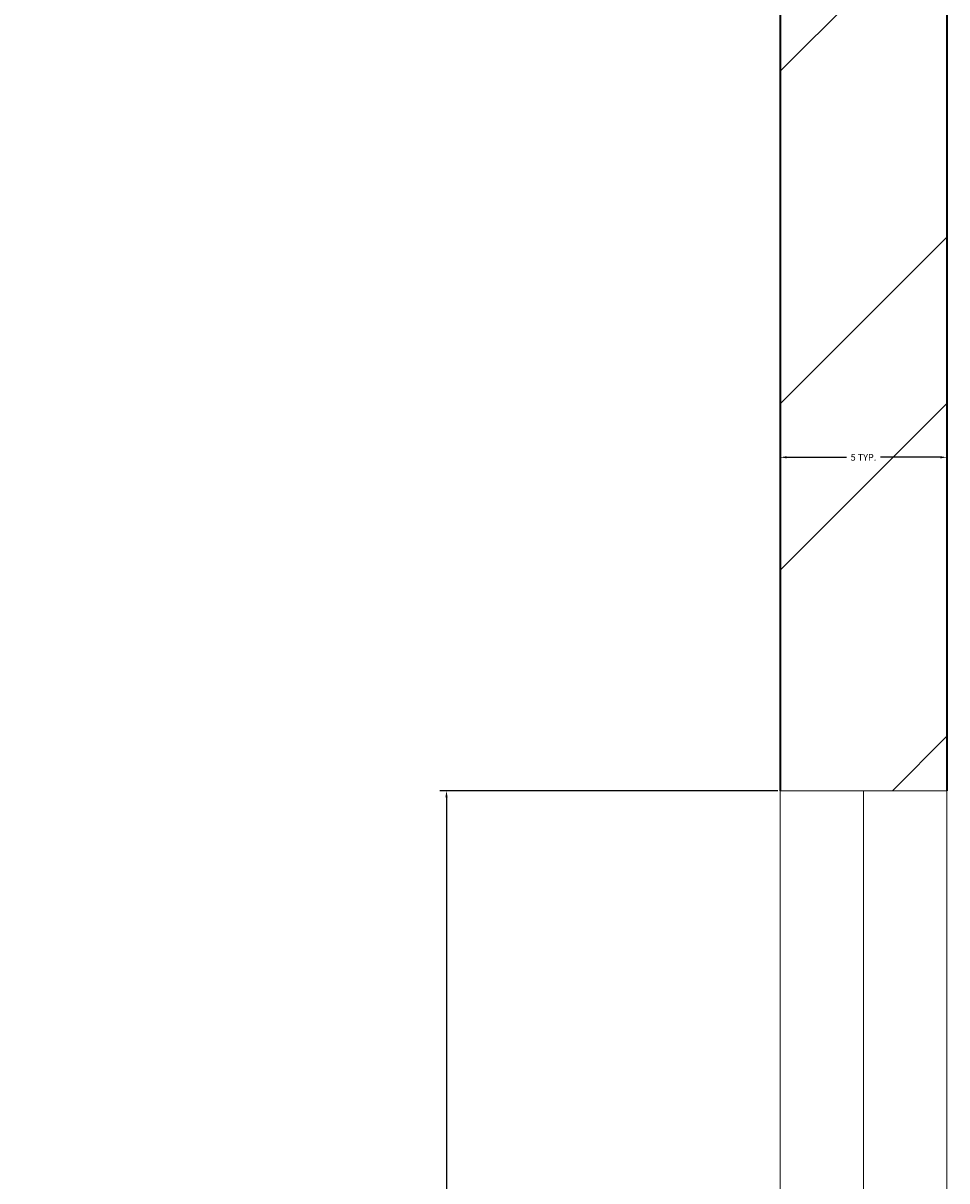
# Model space of a CAD drawing. Units: inches. Extents: x 1885 to 2748, y 783 to 2421.
# Tile 105 of 117: x 2593 to 2618, y 1946 to 1977. Entities that reach past the tile are written whole.
import ezdxf

# ---------------------------------------------------------------- set-up
doc = ezdxf.new("R2010")
doc.units = ezdxf.units.IN
for name, color, linetype, lineweight in [('A-ANNO-DIMS', 2, 'Continuous', 18), ('A-GLAZ', 181, 'Continuous', 18), ('A-WALL', 7, 'Continuous', 35)]:
    doc.layers.add(name, color=color, linetype=linetype, lineweight=lineweight)
doc.layers.add('A-WALL-PATT', color=85, linetype='Continuous', lineweight=13, true_color=0x58ba48)
doc.styles.get("Standard").update_dxf_attribs({"font": 'arial.ttf'})
doc.dimstyles.get("Standard").update_dxf_attribs({"dimtxt": 0.18, "dimasz": 0.18, "dimexe": 0.18, "dimexo": 0.0625, "dimgap": 0.09, "dimtad": 0, "dimtih": 1, "dimtoh": 1, "dimdec": 4, "dimzin": 0, "dimdsep": 46, "dimtxsty": 'Standard', "dimcen": 0.09, "dimadec": 0, "dimazin": 0, "dimtfac": 1, "dimtdec": 4, "dimtofl": 0, "dimtmove": 0, "dimatfit": 3, "dimfxl": 1, "dimtolj": 1, "dimtzin": 0, "dimarcsym": 0})

# ---------------------------------------------------------------- blocks, each defined once
blk = doc.blocks.new('WIN-60-ALT')
for p, q in [((0.004, 59.998), (4.504, 59.998)), ((0.004, 59.998), (0.004, -0.002)), ((4.504, 59.998), (2.254, 59.998)), ((2.254, 59.998), (2.254, -0.002)), ((4.504, -0.002), (4.504, 59.998))]:
    blk.add_line(p, q)
blk = doc.blocks.new('*D17')
at = {"layer": 'A-ANNO-DIMS', "color": 0, "lineweight": -2, "transparency": 16777216}
for p, q in [((2613.711, 1956.755), (2604.594, 1956.755)), ((2604.774, 1956.575), (2604.774, 1926.938)), ((2604.774, 1896.935), (2604.774, 1926.572)), ((2613.711, 1896.755), (2604.594, 1896.755))]:
    blk.add_line(p, q, dxfattribs=at)
at = {"layer": 'A-ANNO-DIMS', "color": 0, "transparency": 16777216}
for points in [[(2604.744, 1956.575), (2604.804, 1956.575), (2604.774, 1956.755)], [(2604.744, 1896.935), (2604.804, 1896.935), (2604.774, 1896.755)]]:
    blk.add_solid(points, dxfattribs=at)
at = {"layer": 'Defpoints', "color": 0, "transparency": 16777216}
for p in [(2604.774, 1956.755), (2613.774, 1956.755), (2613.774, 1896.755)]:
    blk.add_point(p, dxfattribs=at)
at = {"layer": 'A-ANNO-DIMS', "color": 0, "transparency": 16777216, "insert": (2604.774, 1926.755), "char_height": 0.18, "attachment_point": 5}
blk.add_mtext('\\A1;ALT. WINDOW 60 TYP.', dxfattribs=at)
blk = doc.blocks.new('*D18')
at = {"layer": 'A-ANNO-DIMS', "color": 0, "lineweight": -2, "transparency": 16777216}
for p, q in [((2613.774, 1956.817), (2613.774, 1965.935)), ((2618.274, 1956.817), (2618.274, 1965.935)), ((2613.954, 1965.755), (2615.565, 1965.755)), ((2618.094, 1965.755), (2616.482, 1965.755))]:
    blk.add_line(p, q, dxfattribs=at)
at = {"layer": 'A-ANNO-DIMS', "color": 0, "transparency": 16777216}
for points in [[(2613.954, 1965.785), (2613.954, 1965.725), (2613.774, 1965.755)], [(2618.094, 1965.785), (2618.094, 1965.725), (2618.274, 1965.755)]]:
    blk.add_solid(points, dxfattribs=at)
at = {"layer": 'Defpoints', "color": 0, "transparency": 16777216}
for p in [(2618.274, 1965.755), (2613.774, 1956.755), (2618.274, 1956.755)]:
    blk.add_point(p, dxfattribs=at)
at = {"layer": 'A-ANNO-DIMS', "color": 0, "transparency": 16777216, "insert": (2616.024, 1965.755), "char_height": 0.18, "attachment_point": 5}
blk.add_mtext('\\A1;5 TYP.', dxfattribs=at)

msp = doc.modelspace()

# ---------------------------------------------------------------- hatches: boundary and pattern name
at = {"layer": 'A-WALL-PATT'}
h = msp.add_hatch(dxfattribs=at)
h.set_pattern_fill('ANSI32', color=256)
h.paths.add_polyline_path([(2007.772, 2318.006), (1980.774, 2318.006), (1980.774, 2281.215), (1985.274, 2281.215), (1985.274, 2313.506), (2007.772, 2313.506), (2007.772, 2315.756)])
h.paths.add_polyline_path([(2094.324, 2318.006), (2067.772, 2318.006), (2067.772, 2313.506), (2094.324, 2313.506), (2094.324, 2315.756)])
h.paths.add_polyline_path([(2131.367, 2315.756), (2131.367, 2318.006), (2131.189, 2318.006), (2112.609, 2318.006), (2112.609, 2313.506), (2117.274, 2313.506), (2117.274, 2255.201), (2121.774, 2255.201), (2121.774, 2313.506), (2131.367, 2313.506)])
h.paths.add_polyline_path([(2190.512, 2318.006), (2155.367, 2318.006), (2155.367, 2313.506), (2169.774, 2313.506), (2169.774, 2229.506), (2121.774, 2229.506), (2121.774, 2233.451), (2119.524, 2233.451), (2117.274, 2233.451), (2117.274, 2201.101), (2121.774, 2201.101), (2121.774, 2225.006), (2169.774, 2225.006), (2169.774, 2165.006), (2306.274, 2165.006), (2306.274, 2066.006), (2310.774, 2066.006), (2344.274, 2066.006), (2486.274, 2066.006), (2486.274, 1886.006), (2483.02, 1886.006), (2483.02, 1881.506), (2486.274, 1881.506), (2486.274, 1880.678), (2490.774, 1880.678), (2490.774, 2070.506), (2344.274, 2070.506), (2310.774, 2070.506), (2310.774, 2165.006), (2310.774, 2173.636), (2308.524, 2173.636), (2306.274, 2173.636), (2306.274, 2169.506), (2174.274, 2169.506), (2174.274, 2313.506), (2190.512, 2313.506), (2190.512, 2315.756)])
h.paths.add_polyline_path([(1985.274, 2221.215), (1980.774, 2221.215), (1980.774, 2165.006), (1992.774, 2165.006), (1992.774, 2141.927), (1997.274, 2141.927), (1997.274, 2165.006), (2117.274, 2165.006), (2117.274, 2163.126), (2121.774, 2163.126), (2121.774, 2172.734), (2119.524, 2172.734), (2117.274, 2172.734), (2117.274, 2169.506), (1985.274, 2169.506)])
h.paths.add_polyline_path([(1997.274, 2105.927), (1992.774, 2105.927), (1992.774, 2070.506), (2016.774, 2070.506), (2016.774, 2059.123), (2019.024, 2059.123), (2021.274, 2059.123), (2021.274, 2070.506), (2117.274, 2070.506), (2117.274, 2022.506), (2114.423, 2022.506), (2114.423, 2018.006), (2123.627, 2018.006), (2123.627, 2020.256), (2123.627, 2022.506), (2121.774, 2022.506), (2121.774, 2142.587), (2119.524, 2142.587), (2117.274, 2142.587), (2117.274, 2075.006), (1997.274, 2075.006)])
h.paths.add_polyline_path([(2092.029, 2020.256), (2092.029, 2022.506), (2021.274, 2022.506), (2021.274, 2035.123), (2016.774, 2035.123), (2016.774, 2018.006), (2016.774, 1978.784), (2021.274, 1978.784), (2021.274, 2018.006), (2092.029, 2018.006)])
h.paths.add_polyline_path([(2260.938, 2022.506), (2153.105, 2022.506), (2153.105, 2020.256), (2153.105, 2018.006), (2155.274, 2018.006), (2155.274, 1886.006), (2107.629, 1886.006), (2107.629, 1881.506), (2182.911, 1881.506), (2182.911, 1883.756), (2182.911, 1886.006), (2159.774, 1886.006), (2159.774, 2018.006), (2260.938, 2018.006), (2260.938, 2020.256)])
h.paths.add_polyline_path([(2047.629, 1883.756), (2047.629, 1886.006), (2021.274, 1886.006), (2021.274, 1918.784), (2019.024, 1918.784), (2016.774, 1918.784), (2016.774, 1881.506), (2047.629, 1881.506)])
h.paths.add_polyline_path([(2306.361, 1883.756), (2306.361, 1886.006), (2296.274, 1886.006), (2296.274, 1982.006), (2316.535, 1982.006), (2316.535, 1984.256), (2316.535, 1986.506), (2296.274, 1986.506), (2296.274, 2022.506), (2289.276, 2022.506), (2289.276, 2018.006), (2291.774, 2018.006), (2291.774, 1886.006), (2242.911, 1886.006), (2242.911, 1881.506), (2306.361, 1881.506)], flags=17)
h.paths.add_polyline_path([(1985.274, 1843.006), (2021.6, 1843.006), (2021.534, 1845.441), (2021.477, 1847.506), (1980.774, 1847.506), (1980.774, 1809.446), (1985.274, 1809.446)])
h.paths.add_polyline_path([(2131.482, 1845.256), (2131.482, 1847.506), (2081.534, 1847.506), (2081.534, 1843.006), (2117.274, 1843.006), (2117.274, 1784.147), (2119.524, 1784.147), (2121.774, 1784.147), (2121.774, 1843.006), (2131.482, 1843.006)])
h.paths.add_polyline_path([(2203.886, 1847.506), (2155.482, 1847.506), (2155.482, 1843.006), (2169.774, 1843.006), (2169.774, 1759.006), (2121.774, 1759.006), (2121.774, 1761.457), (2117.274, 1761.457), (2117.274, 1730.429), (2121.774, 1730.429), (2121.774, 1754.506), (2177.421, 1754.506), (2177.421, 1756.756), (2177.421, 1759.006), (2174.274, 1759.006), (2174.274, 1843.006), (2203.886, 1843.006)])
h.paths.add_polyline_path([(2335.554, 1845.256), (2335.554, 1847.506), (2239.886, 1847.506), (2239.886, 1843.006), (2306.274, 1843.006), (2306.274, 1759.006), (2199.486, 1759.006), (2199.486, 1754.506), (2310.774, 1754.506), (2310.774, 1843.006), (2335.554, 1843.006)])
h.paths.add_polyline_path([(2348.774, 2022.506), (2344.274, 2022.506), (2344.274, 1986.506), (2341.681, 1986.506), (2341.681, 1982.006), (2344.274, 1982.006), (2344.274, 1886.006), (2330.361, 1886.006), (2330.361, 1881.506), (2361.627, 1881.506), (2361.627, 1883.756), (2361.627, 1886.006), (2348.774, 1886.006)], flags=17)
h.paths.add_polyline_path([(2283.251, 2315.756), (2283.251, 2318.006), (2238.512, 2318.006), (2238.512, 2313.506), (2283.251, 2313.506)], flags=17)
h.paths.add_polyline_path([(2363.274, 2348.006), (2388.677, 2348.006), (2388.677, 2350.256), (2388.677, 2352.506), (2358.774, 2352.506), (2358.774, 2348.006), (2358.774, 2318.006), (2344.481, 2318.006), (2344.481, 2313.506), (2358.774, 2313.506), (2358.774, 2229.506), (2310.774, 2229.506), (2310.774, 2231.952), (2306.274, 2231.952), (2306.274, 2205.611), (2310.774, 2205.611), (2310.774, 2225.006), (2358.774, 2225.006), (2358.774, 2211.506), (2452.329, 2211.506), (2452.329, 2213.756), (2452.329, 2216.006), (2363.274, 2216.006), (2363.274, 2318.006)])
h.paths.add_polyline_path([(2310.774, 2313.506), (2320.481, 2313.506), (2320.481, 2315.756), (2320.481, 2318.006), (2302.728, 2318.006), (2302.728, 2313.506), (2306.274, 2313.506), (2306.274, 2251.076), (2310.774, 2251.076)], flags=17)
h.paths.add_polyline_path([(2490.774, 2352.506), (2486.274, 2352.506), (2448.677, 2352.506), (2448.677, 2348.006), (2486.274, 2348.006), (2486.274, 2318.006), (2486.274, 2216.006), (2481.78, 2216.006), (2481.78, 2211.506), (2486.274, 2211.506), (2486.274, 2165.006), (2493.289, 2165.006), (2493.289, 2167.256), (2493.289, 2169.506), (2490.774, 2169.506), (2490.774, 2313.506), (2494.429, 2313.506), (2494.429, 2318.006), (2490.774, 2318.006)])
h.paths.add_polyline_path([(2534.653, 2318.006), (2515.691, 2318.006), (2515.691, 2313.506), (2534.653, 2313.506), (2534.653, 2315.756)])
h.paths.add_polyline_path([(2618.274, 2318.006), (2594.653, 2318.006), (2594.653, 2313.506), (2613.774, 2313.506), (2613.774, 2281.706), (2618.274, 2281.706)])
h.paths.add_polyline_path([(2618.274, 2221.706), (2613.774, 2221.706), (2613.774, 2169.506), (2554.019, 2169.506), (2554.019, 2165.006), (2613.774, 2165.006), (2613.774, 2152.878), (2618.274, 2152.878)])
h.paths.add_polyline_path([(2618.274, 2128.878), (2616.024, 2128.878), (2613.774, 2128.878), (2613.774, 2117.006), (2529.774, 2117.006), (2529.774, 2165.006), (2532.848, 2165.006), (2532.848, 2169.506), (2522.867, 2169.506), (2522.867, 2165.006), (2525.274, 2165.006), (2525.274, 2117.006), (2525.274, 2112.506), (2525.274, 2108.576), (2529.774, 2108.576), (2529.774, 2112.506), (2613.774, 2112.506), (2613.774, 2080.19), (2618.274, 2080.19)])
h.paths.add_polyline_path([(2618.274, 2044.19), (2616.024, 2044.19), (2613.774, 2044.19), (2613.774, 2015.506), (2529.774, 2015.506), (2529.774, 2088.582), (2527.524, 2088.582), (2525.274, 2088.582), (2525.274, 2011.006), (2613.774, 2011.006), (2613.774, 1956.755), (2618.274, 1956.755)])
h.paths.add_polyline_path([(2618.274, 1881.506), (2618.274, 1896.755), (2613.774, 1896.755), (2613.774, 1881.506), (2613.774, 1847.506), (2592.715, 1847.506), (2592.715, 1843.006), (2613.774, 1843.006), (2613.774, 1765.006), (2613.774, 1760.506), (2609.621, 1760.506), (2609.621, 1756.006), (2613.774, 1756.006), (2613.774, 1660.006), (2608.544, 1660.006), (2608.544, 1655.506), (2613.774, 1655.506), (2613.774, 1508.158), (2618.274, 1508.158)])
h.paths.add_polyline_path([(2565.774, 1843.006), (2568.997, 1843.006), (2568.997, 1847.506), (2490.774, 1847.506), (2490.774, 1849.7), (2488.524, 1849.7), (2486.274, 1849.7), (2486.274, 1847.506), (2477.274, 1847.506), (2477.274, 1838.506), (2477.274, 1821.493), (2486.274, 1821.493), (2486.274, 1838.506), (2561.274, 1838.506), (2561.274, 1765.006), (2486.274, 1765.006), (2486.274, 1786.157), (2477.274, 1786.157), (2477.274, 1765.006), (2477.274, 1756.006), (2486.274, 1756.006), (2565.774, 1756.006), (2585.621, 1756.006), (2585.621, 1758.256), (2585.621, 1760.506), (2565.774, 1760.506), (2565.774, 1765.006)])
h.paths.add_polyline_path([(2486.274, 1651.006), (2561.274, 1651.006), (2561.274, 1567.006), (2486.274, 1567.006), (2486.274, 1591.321), (2477.274, 1591.321), (2477.274, 1567.006), (2477.274, 1558.006), (2477.274, 1555.439), (2481.774, 1555.439), (2481.774, 1558.006), (2568.653, 1558.006), (2568.653, 1560.256), (2568.653, 1562.506), (2565.774, 1562.506), (2565.774, 1655.506), (2584.544, 1655.506), (2584.544, 1657.756), (2584.544, 1660.006), (2565.774, 1660.006), (2486.274, 1660.006), (2477.274, 1660.006), (2477.274, 1651.006), (2477.274, 1632.989), (2486.274, 1632.989)])
h.paths.add_polyline_path([(2449.967, 1883.756), (2449.967, 1886.006), (2421.627, 1886.006), (2421.627, 1881.506), (2449.967, 1881.506)], flags=17)
h.paths.add_polyline_path([(2447.274, 1847.506), (2395.554, 1847.506), (2395.554, 1843.006), (2442.774, 1843.006), (2442.774, 1809.27), (2447.274, 1809.27)])
h.paths.add_polyline_path([(1985.274, 1749.446), (1980.774, 1749.446), (1980.774, 1694.504), (1985.274, 1694.504), (1985.274, 1694.506), (1986.897, 1694.506), (1986.897, 1697.78), (1986.897, 1699.006), (1985.274, 1699.006)])
h.paths.add_polyline_path([(2152.774, 1699.006), (2121.774, 1699.006), (2121.774, 1703.668), (2119.524, 1703.668), (2117.274, 1703.668), (2117.274, 1699.006), (2009.219, 1699.006), (2009.219, 1694.506), (2148.274, 1694.506), (2148.274, 1692.631), (2152.774, 1692.631)])
h.paths.add_polyline_path([(2016.274, 1694.506), (2011.774, 1694.506), (2011.774, 1558.006), (2040.806, 1558.006), (2040.806, 1560.256), (2040.806, 1562.506), (2016.274, 1562.506)])
h.paths.add_polyline_path([(2152.774, 1663.017), (2150.524, 1663.017), (2148.274, 1663.017), (2148.274, 1562.506), (2100.806, 1562.506), (2100.806, 1558.006), (2165.119, 1558.006), (2165.119, 1560.256), (2165.119, 1562.506), (2152.774, 1562.506), (2152.774, 1610.506), (2224.774, 1610.506), (2224.774, 1607.99), (2229.274, 1607.99), (2229.274, 1615.006), (2152.774, 1615.006)])
h.paths.add_polyline_path([(2238.613, 1560.256), (2238.613, 1562.506), (2229.274, 1562.506), (2229.274, 1588.756), (2227.024, 1588.763), (2224.774, 1588.771), (2224.774, 1562.506), (2189.119, 1562.506), (2189.119, 1558.006), (2238.613, 1558.006)])
h.paths.add_polyline_path([(2336.024, 1560.256), (2336.024, 1562.506), (2310.774, 1562.506), (2310.774, 1656.347), (2308.524, 1656.347), (2306.274, 1656.347), (2306.274, 1562.506), (2286.613, 1562.506), (2286.613, 1558.006), (2336.024, 1558.006)])
h.paths.add_polyline_path([(2447.274, 1690.968), (2445.024, 1690.968), (2442.774, 1690.968), (2442.774, 1687.006), (2306.274, 1687.006), (2306.274, 1680.75), (2310.774, 1680.75), (2310.774, 1682.506), (2442.774, 1682.506), (2442.774, 1562.506), (2396.024, 1562.506), (2396.024, 1558.006), (2447.274, 1558.006)])
h.paths.add_polyline_path([(2447.274, 1749.27), (2445.024, 1749.27), (2442.774, 1749.27), (2442.774, 1717.232), (2447.274, 1717.232)])
h.paths.add_polyline_path([(2044.674, 1521.756), (2044.674, 1524.006), (2007.274, 1524.006), (2007.274, 1503.49), (2009.524, 1503.49), (2011.774, 1503.49), (2011.774, 1519.506), (2044.674, 1519.506)])
h.paths.add_polyline_path([(2177.969, 1521.756), (2177.969, 1524.006), (2104.674, 1524.006), (2104.674, 1519.506), (2145.774, 1519.506), (2145.774, 1387.506), (2143.37, 1387.506), (2143.37, 1383.006), (2251.585, 1383.006), (2251.585, 1385.256), (2251.585, 1387.506), (2150.274, 1387.506), (2150.274, 1519.506), (2177.969, 1519.506)])
h.paths.add_polyline_path([(2298.704, 1524.006), (2237.969, 1524.006), (2237.969, 1519.506), (2282.274, 1519.506), (2282.274, 1387.506), (2279.683, 1387.506), (2279.683, 1383.006), (2286.774, 1383.006), (2286.774, 1419.006), (2312.451, 1419.006), (2312.451, 1421.256), (2312.451, 1423.506), (2286.774, 1423.506), (2286.774, 1519.506), (2298.704, 1519.506), (2298.704, 1521.722)], flags=17)
h.paths.add_polyline_path([(2361.897, 1521.756), (2361.897, 1524.006), (2322.704, 1524.006), (2322.704, 1519.506), (2334.774, 1519.506), (2334.774, 1423.506), (2331.93, 1423.506), (2331.93, 1419.006), (2334.774, 1419.006), (2334.774, 1387.506), (2334.774, 1383.228), (2339.274, 1383.228), (2339.274, 1387.506), (2339.274, 1519.506), (2361.897, 1519.506)], flags=17)
h.paths.add_polyline_path([(2447.274, 1521.756), (2447.274, 1524.006), (2421.897, 1524.006), (2421.897, 1519.506), (2447.274, 1519.506)], flags=17)
h.paths.add_polyline_path([(2481.774, 1529.6), (2479.524, 1529.6), (2477.274, 1529.6), (2477.274, 1524.006), (2474.489, 1524.006), (2474.489, 1519.506), (2477.274, 1519.506), (2477.274, 1334.506), (2296.774, 1334.506), (2296.774, 1240.506), (2160.274, 1240.506), (2160.274, 1180.506), (2112.274, 1180.506), (2112.274, 1207.692), (2110.024, 1207.692), (2107.774, 1207.692), (2107.774, 1171.609), (2112.274, 1171.609), (2112.274, 1176.006), (2160.274, 1176.006), (2160.274, 1092.006), (2144.221, 1092.006), (2144.221, 1087.506), (2189.497, 1087.506), (2189.497, 1089.756), (2189.497, 1092.006), (2164.774, 1092.006), (2164.774, 1236.006), (2296.774, 1236.006), (2296.774, 1231.912), (2301.274, 1231.912), (2301.274, 1330.006), (2481.774, 1330.006), (2481.774, 1387.506)])
h.paths.add_polyline_path([(2618.274, 1448.158), (2613.774, 1448.158), (2613.774, 1382.506), (2529.774, 1382.506), (2525.274, 1382.506), (2525.274, 1307.062), (2529.774, 1307.062), (2529.774, 1378.006), (2613.774, 1378.006), (2613.774, 1354.988), (2618.274, 1354.988)])
h.paths.add_polyline_path([(2618.274, 1318.988), (2613.774, 1318.988), (2613.774, 1281.006), (2529.774, 1281.006), (2529.774, 1283.786), (2527.524, 1283.786), (2525.274, 1283.786), (2525.274, 1228.506), (2516.794, 1228.506), (2516.794, 1224.006), (2533.484, 1224.006), (2533.484, 1226.256), (2533.484, 1228.506), (2529.774, 1228.506), (2529.774, 1276.506), (2613.774, 1276.506), (2613.774, 1266.02), (2618.274, 1266.02)])
h.paths.add_polyline_path([(2618.274, 1134.964), (2613.774, 1134.964), (2613.774, 1092.006), (2594.545, 1092.006), (2594.545, 1087.506), (2618.274, 1087.506)])
h.paths.add_polyline_path([(2534.545, 1092.006), (2509.765, 1092.006), (2509.765, 1087.506), (2534.545, 1087.506), (2534.545, 1089.756)])
h.paths.add_polyline_path([(2481.274, 1224.006), (2484.117, 1224.006), (2484.117, 1226.256), (2484.117, 1228.506), (2476.774, 1228.506), (2476.774, 1198.506), (2471.61, 1198.506), (2471.61, 1194.006), (2476.774, 1194.006), (2476.774, 1062.006), (2436.894, 1062.006), (2436.894, 1057.506), (2476.774, 1057.506), (2481.274, 1057.506), (2481.274, 1062.006), (2481.274, 1087.506), (2485.354, 1087.506), (2485.354, 1089.756), (2485.354, 1092.006), (2481.274, 1092.006), (2481.274, 1117.506)])
h.paths.add_polyline_path([(2439.898, 1198.506), (2349.274, 1198.506), (2349.274, 1194.006), (2349.274, 1180.506), (2301.274, 1180.506), (2301.274, 1201.896), (2299.024, 1201.896), (2296.774, 1201.896), (2296.774, 1172.335), (2299.024, 1172.335), (2301.274, 1172.335), (2301.274, 1176.006), (2349.274, 1176.006), (2349.274, 1092.006), (2334.452, 1092.006), (2334.452, 1087.506), (2349.274, 1087.506), (2349.274, 1057.506), (2353.774, 1057.506), (2376.894, 1057.506), (2376.894, 1059.756), (2376.894, 1062.006), (2353.774, 1062.006), (2353.774, 1087.506), (2353.774, 1180.506), (2353.774, 1194.006), (2439.898, 1194.006), (2439.898, 1196.256)])
h.paths.add_polyline_path([(2270.596, 1089.756), (2270.596, 1092.006), (2249.497, 1092.006), (2249.497, 1087.506), (2270.596, 1087.506)], flags=17)
h.paths.add_polyline_path([(2310.452, 1092.006), (2301.274, 1092.006), (2301.274, 1153.292), (2296.774, 1153.292), (2296.774, 1092.006), (2293.786, 1092.006), (2293.786, 1087.506), (2310.452, 1087.506), (2310.452, 1089.756)], flags=17)
h.paths.add_polyline_path([(2112.274, 1150.328), (2110.024, 1150.328), (2107.774, 1150.328), (2107.774, 1092.006), (2104.465, 1092.006), (2104.465, 1087.506), (2120.221, 1087.506), (2120.221, 1089.756), (2120.221, 1092.006), (2112.274, 1092.006)])
h.paths.add_polyline_path([(2082.172, 1092.006), (2058.144, 1092.006), (2058.144, 1087.506), (2082.172, 1087.506), (2082.172, 1089.756)])
h.paths.add_polyline_path([(1975.774, 1145.638), (1971.274, 1145.638), (1971.274, 1087.506), (1980.774, 1087.506), (1998.144, 1087.506), (1998.144, 1089.756), (1998.144, 1092.006), (1985.274, 1092.006), (1975.774, 1092.006)])
h.paths.add_polyline_path([(2112.274, 1244.385), (2110.024, 1244.385), (2107.774, 1244.385), (2107.774, 1240.506), (1992.274, 1240.506), (1992.274, 1271.008), (1987.774, 1271.008), (1987.774, 1240.506), (1980.774, 1240.506), (1975.774, 1240.506), (1971.274, 1240.506), (1971.274, 1205.638), (1975.774, 1205.638), (1975.774, 1236.006), (2107.774, 1236.006), (2107.774, 1233.444), (2112.274, 1233.444), (2112.274, 1236.006)])
h.paths.add_polyline_path([(2112.274, 1383.006), (2114.783, 1383.006), (2114.783, 1385.256), (2114.783, 1387.506), (2102.476, 1387.506), (2102.476, 1383.006), (2107.774, 1383.006), (2107.774, 1335.006), (2011.774, 1335.006), (2011.774, 1349.939), (2007.274, 1349.939), (2007.274, 1335.006), (1987.774, 1335.006), (1987.774, 1330.506), (1987.774, 1307.008), (1992.274, 1307.008), (1992.274, 1330.506), (2007.274, 1330.506), (2107.774, 1330.506), (2107.774, 1264.711), (2112.274, 1264.711)])
h.paths.add_polyline_path([(2077.857, 1387.506), (2011.774, 1387.506), (2011.774, 1390.036), (2009.524, 1390.036), (2007.274, 1390.036), (2007.274, 1373.939), (2011.774, 1373.939), (2011.774, 1383.006), (2077.857, 1383.006)])
h.paths.add_polyline_path([(2011.774, 1443.49), (2007.274, 1443.49), (2007.274, 1410.248), (2011.774, 1410.248)])

# ---------------------------------------------------------------- linework, layer by layer
at = {"layer": 'A-WALL'}
for p, q in [((2618.274, 2044.19), (2618.274, 1956.755)), ((2613.774, 2011.006), (2613.774, 1956.755))]:
    msp.add_line(p, q, dxfattribs=at)

# ---------------------------------------------------------------- block references
at = {"layer": 'A-GLAZ'}
msp.add_blockref('WIN-60-ALT', (2613.77, 1896.757), dxfattribs=at)

# ---------------------------------------------------------------- dimensions: what is measured, and where the dimension line sits
at = {"layer": 'A-ANNO-DIMS'}
dim = msp.add_linear_dim(base=(2618.273597599, 1965.75492547), p1=(2613.773597599, 1956.75492547), p2=(2618.273597599, 1956.75492547), text='<> TYP.', dimstyle='Standard', override={"dimdec": 0, "dimlfac": 1, "dimrnd": 0, "dimzin": 0, "dimdsep": 46, "dimlunit": 2}, dxfattribs=at)
dim.commit()
dim.dimension.update_dxf_attribs({"geometry": '*D18', "text_midpoint": (2616.023597599, 1965.75492547)})
dim = msp.add_linear_dim(base=(2604.774, 1956.755), p1=(2613.774, 1896.755), p2=(2613.774, 1956.755), angle=90, text='ALT. WINDOW <> TYP.', dimstyle='Standard', override={"dimdec": 0, "dimlfac": 1, "dimrnd": 0, "dimzin": 0, "dimdsep": 46, "dimlunit": 2}, dxfattribs=at)
dim.commit()
dim.dimension.update_dxf_attribs({"geometry": '*D17', "text_midpoint": (2604.774, 1926.755)})

doc.saveas('drawing.dxf')
